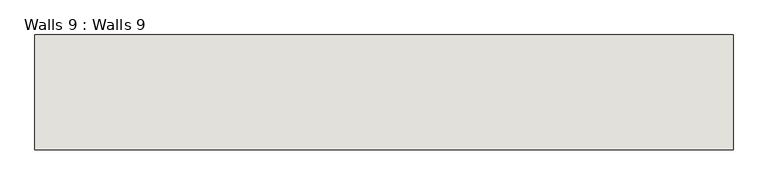
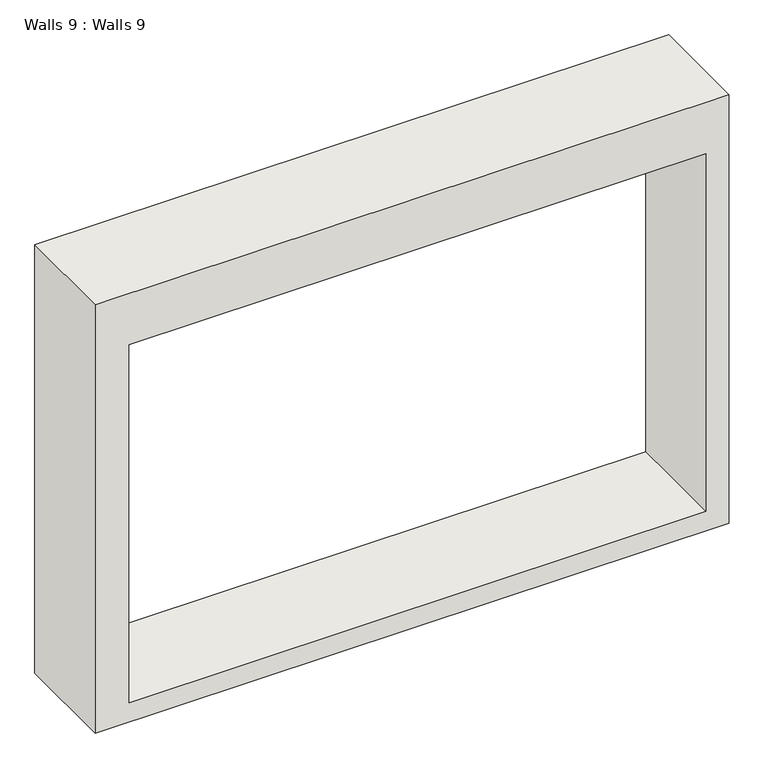
"""IFC4 building model written with IfcOpenShell, lengths in millimetres: wall geometry, Walls 9 : Walls 9."""

from ifc_helpers import new_model, si_unit, frame, origin, place, context, project, spatial, polyline, outline, extrude, source, transform, mapped, element, save


def walls_9_walls_9_e6c342de(model_context):
    return source(origin(), model_context, "Body", "SweptSolid", [
        extrude(outline(polyline([(3048.0, -9880.3407032), (3048.0, -6171.9407032), (5696.0, -6171.9407032), (5696.0, -9880.3407032), (3048.0, -9880.3407032)]), holes=[polyline([(3166.8390699, -9680.3407032), (5378.7951143, -9680.3407032), (5378.7951143, -6306.4066261), (3166.8390699, -6306.4066261), (3166.8390699, -9680.3407032)])]), frame((0.0, 3251.3956099, 0.0), z_axis=(0.0, 1.0, 0.0), x_axis=(0.0, 0.0, 1.0)), (0.0, 0.0, 1.0), 609.6),
    ])


if __name__ == "__main__":
    model = new_model("IFC4")
    model_context = context("Model", 3, world=origin())
    ifc_project = project(units=[si_unit("LENGTHUNIT", "METRE", prefix="MILLI")], contexts=[model_context])
    site = spatial("IfcSite", under=ifc_project)
    building = spatial("IfcBuilding", under=site)
    placement = place(None, origin())
    walls_9_walls_9_shape = walls_9_walls_9_e6c342de(model_context)
    element("IfcWall", 1, ObjectType="Walls 9 : Walls 9", at=placement, inside=building, context=model_context, shape_type="MappedRepresentation", body=[
        mapped(walls_9_walls_9_shape, transform((0.0, 0.0, 0.0), x_axis=(1.0, 0.0, 0.0), y_axis=(0.0, 1.0, 0.0), z_axis=(0.0, 0.0, 1.0))),
    ])
    save(model, "model.ifc")

# Revit data of these elements
# Element 1 (IfcWall, "Walls 9 : Walls 9")
#   Materials on its faces: "Default Wall"
# Materials
#   "Default Wall": colour RGB 80 80 80, transparency 0
